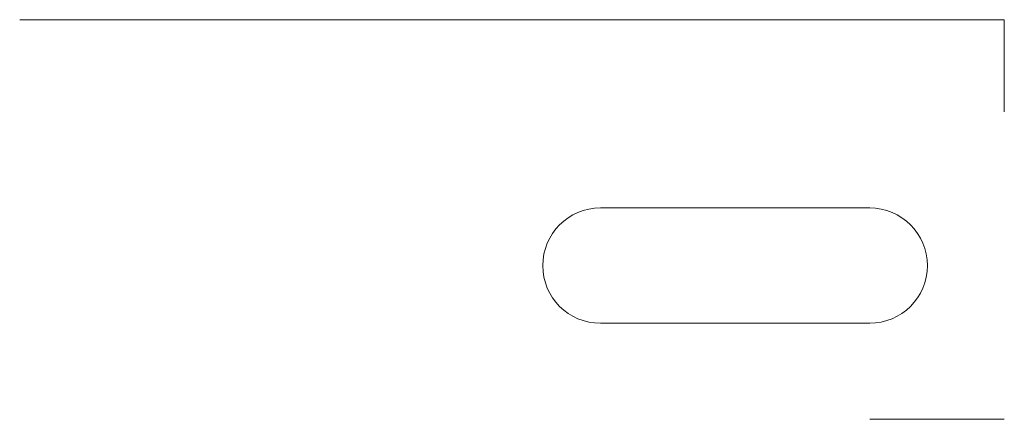
# Model space of a CAD drawing. Units: millimetres. Extents: x 82 to 210, y -52 to 786.
# Tile 1 of 1: x 81.8 to 209.8, y -52 to 0. Entities that reach past the tile are written whole.
import ezdxf

# ---------------------------------------------------------------- set-up
doc = ezdxf.new("R2010")
doc.units = ezdxf.units.MM
doc.layers.add('M-CONS', color=8, linetype='Continuous', lineweight=18)

msp = doc.modelspace()

# ---------------------------------------------------------------- linework, layer by layer
at = {"layer": 'M-CONS'}
msp.add_line((209.82, -52, 10.21), (192.32, -52, 10.21), dxfattribs=at)
at = {"layer": 'M-CONS', "extrusion": (0, -1, 0)}
msp.add_lwpolyline([(141.82, 10.21), (141.82, 25.21, 1), (81.82, 25.21), (81.82, -4.79), (141.82, -4.79)], format="xyb", dxfattribs=at)
msp.add_lwpolyline([(81.82, -4.79), (209.82, -4.79), (209.82, 10.21)], dxfattribs=at)
at = {"layer": 'M-CONS', "extrusion": (1, 0, 0), "elevation": 209.82}
msp.add_lwpolyline([(-12, 10.21), (0, 10.21), (-10, 10.21), (-10, -15.79), (0, -15.79), (0, 10.13)], dxfattribs=at)
at = {"layer": 'M-CONS', "elevation": 10.21}
msp.add_lwpolyline([(157.32, -24.5, 1), (157.32, -39.5), (192.32, -39.5, 1), (192.32, -24.5)], format="xyb", close=True, dxfattribs=at)
at = {"layer": 'M-CONS', "extrusion": (0, -1, 0)}
msp.add_circle((111.82, 25.21), 15, dxfattribs=at)

doc.saveas('drawing.dxf')
